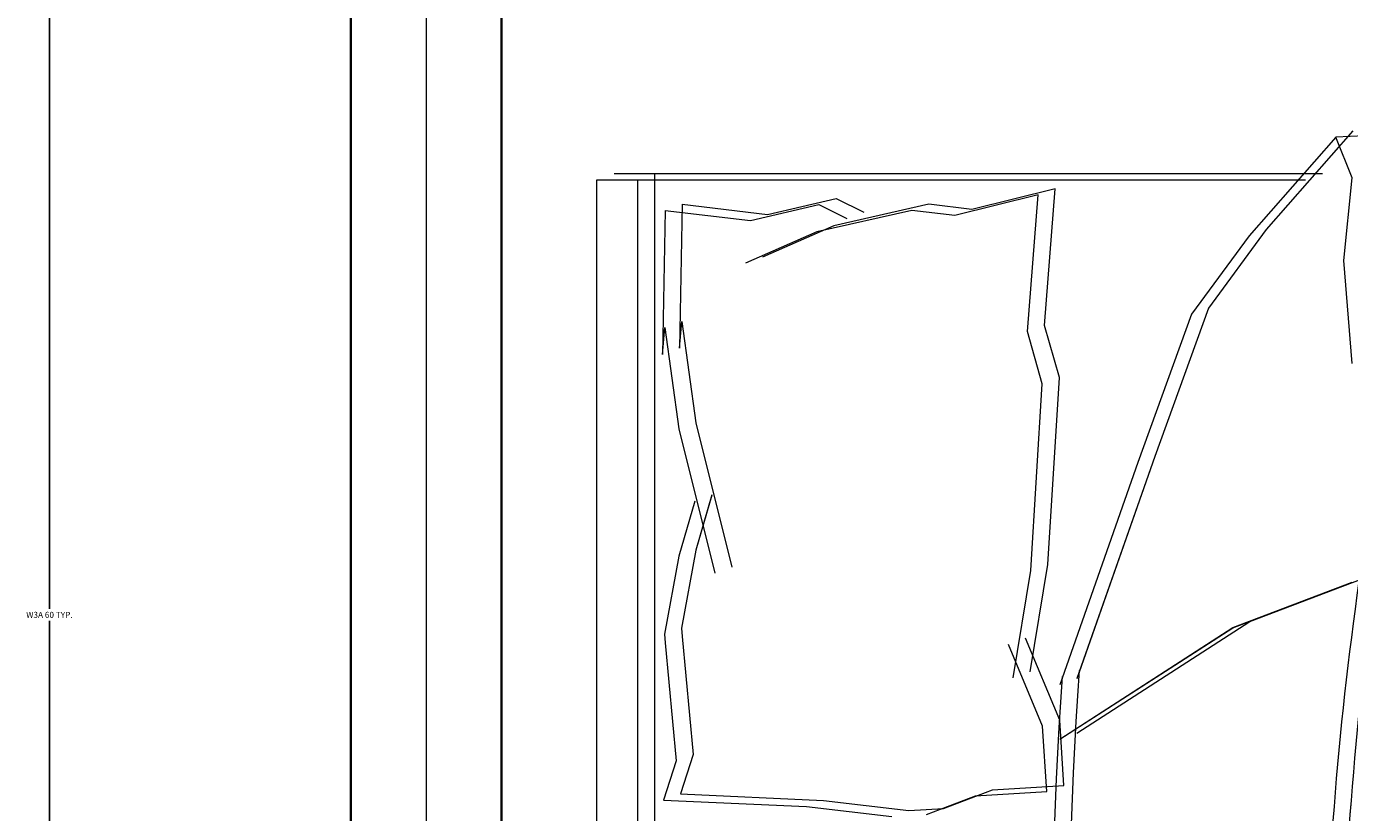
# Model space of a CAD drawing. Units: inches. Extents: x 1962 to 2771, y 1245 to 2660.
# Tile 26 of 114: x 2077 to 2116, y 1871 to 1894. Entities that reach past the tile are written whole.
import ezdxf

# ---------------------------------------------------------------- set-up
doc = ezdxf.new("R2010")
doc.units = ezdxf.units.IN
for name, color, linetype, lineweight in [('A-ANNO-DIMS', 2, 'Continuous', 18), ('A-FURN', 8, 'Continuous', 13), ('A-GLAZ', 4, 'Continuous', 18), ('A-WALL', 7, 'Continuous', 35)]:
    doc.layers.add(name, color=color, linetype=linetype, lineweight=lineweight)
doc.styles.get("Standard").update_dxf_attribs({"font": 'arial.ttf'})
doc.dimstyles.get("Standard").update_dxf_attribs({"dimtxt": 0.18, "dimasz": 0.18, "dimexe": 0.18, "dimexo": 0.0625, "dimgap": 0.09, "dimtad": 0, "dimtih": 1, "dimtoh": 1, "dimdec": 4, "dimzin": 0, "dimdsep": 46, "dimtxsty": 'Standard', "dimcen": 0.09, "dimadec": 0, "dimazin": 0, "dimtfac": 1, "dimtdec": 4, "dimtofl": 0, "dimtmove": 0, "dimatfit": 3, "dimfxl": 1, "dimtolj": 1, "dimtzin": 0, "dimarcsym": 0})

# ---------------------------------------------------------------- blocks, each defined once
blk = doc.blocks.new('BED-PLAN')
for p, q in [((22.055, 42.025), (19.471, 39.08)), ((22.055, 42.025), (19.471, 39.08)), ((22.563, 42.207), (19.979, 39.261)), ((22.563, 42.206), (19.979, 39.261)), ((23.442, 42.088), (22.055, 42.025, 3.077)), ((23.442, 42.088), (22.055, 42.025, 3.077)), ((22.547, 40.803), (22.055, 42.025)), ((22.547, 40.803), (22.055, 42.025)), ((0, 40.752), (21.152, 40.752)), ((0, 40.751), (21.152, 40.751)), ((0, 2.764), (0, 40.751)), ((0.508, 40.933), (21.66, 40.933)), ((0.508, 40.933), (21.66, 40.933)), ((1.219, 2.764), (1.219, 40.752)), ((1.219, 2.763), (1.219, 40.751)), ((1.727, 2.945), (1.727, 40.933)), ((1.727, 2.945), (1.727, 40.933)), ((22.301, 38.341), (22.547, 40.803)), ((22.301, 38.341), (22.547, 40.803)), ((13.173, 40.301), (10.679, 39.684)), ((13.173, 40.301), (10.679, 39.684)), ((13.682, 40.482), (11.187, 39.866)), ((13.682, 40.482), (11.187, 39.866)), ((12.853, 36.222), (13.173, 40.301)), ((12.853, 36.221), (13.173, 40.301)), ((13.361, 36.403), (13.682, 40.482)), ((13.361, 36.403), (13.682, 40.482)), ((2.541, 40.016), (2.464, 35.722)), ((2.541, 40.016), (2.464, 35.722)), ((2.541, 40.016), (5.093, 39.715)), ((2.541, 40.016), (5.093, 39.715)), ((4.585, 39.534), (6.628, 40.007)), ((4.585, 39.533), (6.628, 40.007)), ((5.093, 39.715), (7.136, 40.188)), ((5.093, 39.715), (7.136, 40.188)), ((6.628, 40.007), (7.46, 39.598)), ((6.628, 40.007), (7.46, 39.598)), ((9.911, 40.016), (7.072, 39.378)), ((9.911, 40.016), (7.072, 39.378)), ((7.136, 40.188), (7.968, 39.78)), ((7.136, 40.188), (7.968, 39.78)), ((11.187, 39.866), (9.911, 40.016)), ((11.187, 39.866), (9.911, 40.016)), ((2.033, 39.835), (1.955, 35.54)), ((2.033, 39.834), (1.956, 35.54)), ((2.033, 39.835), (4.585, 39.534)), ((2.033, 39.834), (4.585, 39.533)), ((9.402, 39.835), (6.563, 39.197)), ((9.402, 39.835), (6.563, 39.197)), ((10.679, 39.684), (9.402, 39.835)), ((10.679, 39.684), (9.402, 39.835)), ((6.563, 39.197), (4.434, 38.258)), ((6.563, 39.197), (4.434, 38.258)), ((7.072, 39.378), (4.942, 38.439)), ((7.072, 39.378), (4.942, 38.439)), ((19.979, 39.261), (18.257, 36.922)), ((19.979, 39.261), (18.257, 36.922)), ((19.471, 39.08), (17.749, 36.741)), ((19.471, 39.08), (17.749, 36.741)), ((22.547, 35.263), (22.301, 38.341)), ((22.547, 35.263), (22.301, 38.341)), ((17.749, 36.741), (16.149, 32.309)), ((17.749, 36.741), (16.149, 32.309)), ((18.257, 36.922), (16.658, 32.49)), ((18.257, 36.922), (16.658, 32.49)), ((2.464, 35.722), (2.529, 36.519)), ((2.464, 35.722), (2.529, 36.519)), ((2.529, 36.519), (2.948, 33.5)), ((2.529, 36.519), (2.948, 33.5)), ((13.804, 34.845), (13.361, 36.403)), ((13.804, 34.845), (13.361, 36.403)), ((1.955, 35.54), (2.021, 36.338)), ((1.956, 35.54), (2.021, 36.337)), ((2.021, 36.338), (2.44, 33.319)), ((2.021, 36.337), (2.44, 33.318)), ((13.296, 34.663), (12.853, 36.222)), ((13.296, 34.663), (12.853, 36.221)), ((13.461, 29.273), (13.804, 34.845)), ((13.461, 29.273), (13.804, 34.845)), ((12.953, 29.091), (13.296, 34.663)), ((12.953, 29.091), (13.296, 34.663)), ((2.44, 33.319), (3.515, 29.011)), ((2.44, 33.318), (3.515, 29.011)), ((2.948, 33.5), (4.023, 29.192)), ((2.948, 33.5), (4.023, 29.192)), ((16.658, 32.49), (14.326, 25.863)), ((16.658, 32.49), (14.326, 25.862)), ((16.149, 32.309), (13.818, 25.681)), ((16.149, 32.309), (13.818, 25.681)), ((3.428, 31.343), (2.955, 29.701)), ((3.428, 31.342), (2.955, 29.701)), ((2.92, 31.161), (2.447, 29.52)), ((2.92, 31.161), (2.447, 29.519)), ((2.955, 29.701), (2.525, 27.372)), ((2.955, 29.701), (2.525, 27.372)), ((2.447, 29.52), (2.017, 27.19)), ((2.447, 29.519), (2.017, 27.19)), ((12.931, 26.068), (13.461, 29.273)), ((12.931, 26.068), (13.461, 29.273)), ((12.423, 25.886), (12.953, 29.091)), ((12.423, 25.886), (12.953, 29.091)), ((19.487, 27.566), (23.055, 28.92)), ((19.487, 27.566), (23.055, 28.92)), ((18.979, 27.385), (22.547, 28.739)), ((18.979, 27.384), (22.547, 28.739)), ((2.525, 27.372), (2.541, 27.117)), ((2.525, 27.372), (2.541, 27.116)), ((13.818, 24.054), (18.979, 27.385)), ((13.818, 24.054), (18.979, 27.384)), ((14.326, 24.236), (19.487, 27.566)), ((14.326, 24.235), (19.487, 27.566)), ((2.017, 27.19), (2.033, 26.935)), ((2.017, 27.19), (2.033, 26.935)), ((2.033, 26.935), (2.368, 23.415)), ((2.033, 26.935), (2.368, 23.415)), ((2.541, 27.117), (2.876, 23.597)), ((2.541, 27.116), (2.876, 23.597)), ((13.306, 24.444), (12.285, 26.885)), ((13.306, 24.444), (12.285, 26.885)), ((13.814, 24.626), (12.793, 27.067)), ((13.814, 24.626), (12.793, 27.066)), ((13.936, 22.676), (13.814, 24.626)), ((13.936, 22.676), (13.814, 24.626)), ((13.428, 22.495), (13.306, 24.444)), ((13.428, 22.495), (13.306, 24.444)), ((2.368, 23.415), (1.981, 22.24)), ((2.368, 23.415), (1.981, 22.24)), ((2.876, 23.597), (2.489, 22.421)), ((2.876, 23.597), (2.489, 22.421)), ((10.346, 21.991), (11.809, 22.543)), ((10.346, 21.991), (11.809, 22.543)), ((11.809, 22.543), (13.936, 22.676)), ((11.809, 22.543), (13.936, 22.676)), ((1.981, 22.24), (6.254, 22.046)), ((1.981, 22.24), (6.254, 22.046)), ((2.489, 22.421), (6.762, 22.228)), ((2.489, 22.421), (6.762, 22.228)), ((6.762, 22.228), (9.314, 21.927)), ((6.762, 22.228), (9.314, 21.927)), ((9.838, 21.81), (11.301, 22.362)), ((9.838, 21.81), (11.301, 22.362)), ((11.301, 22.362), (13.428, 22.495)), ((11.301, 22.362), (13.428, 22.495)), ((6.254, 22.046), (8.806, 21.745)), ((6.254, 22.046), (8.806, 21.745)), ((9.314, 21.927), (10.346, 21.991)), ((9.314, 21.927), (10.346, 21.991))]:
    blk.add_line(p, q)
for centre, radius, start, end in [((124.762, 14.297), 102.556, 171.78449, 186.90062), ((124.762, 14.296), 102.556, 171.78449, 186.90062), ((124.254, 14.115), 102.556, 171.78449, 186.90062), ((124.254, 14.115), 102.556, 171.78449, 186.90062), ((145.219, 17.161), 131.131, 176.08655, 186.78213), ((145.219, 17.161), 131.131, 176.08655, 186.78213), ((144.711, 16.979), 131.131, 176.08655, 186.78213), ((144.711, 16.979), 131.131, 176.08655, 186.78213)]:
    blk.add_arc(centre, radius, start, end)
blk = doc.blocks.new('WIN-60IN-A')
blk.add_line((2.25, 60), (2.25, 0))
blk = doc.blocks.new('*D22')
at = {"layer": 'A-ANNO-DIMS', "color": 0, "lineweight": -2, "transparency": 16777216}
for p, q in [((2086.245, 1906.501), (2077.127, 1906.501)), ((2077.307, 1906.321), (2077.307, 1876.683)), ((2077.307, 1846.681), (2077.307, 1876.319)), ((2086.245, 1846.501), (2077.127, 1846.501))]:
    blk.add_line(p, q, dxfattribs=at)
at = {"layer": 'A-ANNO-DIMS', "color": 0, "transparency": 16777216}
for points in [[(2077.277, 1906.321), (2077.337, 1906.321), (2077.307, 1906.501)], [(2077.277, 1846.681), (2077.337, 1846.681), (2077.307, 1846.501)]]:
    blk.add_solid(points, dxfattribs=at)
at = {"layer": 'Defpoints', "color": 0, "transparency": 16777216}
for p in [(2077.307, 1906.501), (2086.307, 1906.501), (2086.307, 1846.501)]:
    blk.add_point(p, dxfattribs=at)
at = {"layer": 'A-ANNO-DIMS', "color": 0, "transparency": 16777216, "insert": (2077.307, 1876.501), "char_height": 0.18, "attachment_point": 5}
blk.add_mtext('\\A1;W3A 60 TYP.', dxfattribs=at)

msp = doc.modelspace()

# ---------------------------------------------------------------- linework, layer by layer
at = {"layer": 'A-WALL'}
for p, q in [((2086.3074, 1928.8437), (2086.3074, 1486.3437)), ((2090.8074, 1928.8437), (2090.8074, 1784.8437))]:
    msp.add_line(p, q, dxfattribs=at)

# ---------------------------------------------------------------- block references
at = {"layer": 'A-FURN'}
msp.add_blockref('BED-PLAN', (2093.6551, 1848.7344), dxfattribs=at)
at = {"layer": 'A-GLAZ'}
msp.add_blockref('WIN-60IN-A', (2086.3074, 1846.5013), dxfattribs=at)

# ---------------------------------------------------------------- dimensions: what is measured, and where the dimension line sits
at = {"layer": 'A-ANNO-DIMS'}
dim = msp.add_linear_dim(base=(2077.3074, 1906.5013), p1=(2086.3074, 1846.5013), p2=(2086.3074, 1906.5013), angle=90, text='W3A <> TYP.', dimstyle='Standard', override={"dimdec": 0, "dimlfac": 1, "dimrnd": 0, "dimzin": 0, "dimdsep": 46, "dimlunit": 2}, dxfattribs=at)
dim.commit()
dim.dimension.update_dxf_attribs({"geometry": '*D22', "text_midpoint": (2077.3074, 1876.5013)})

doc.saveas('drawing.dxf')
